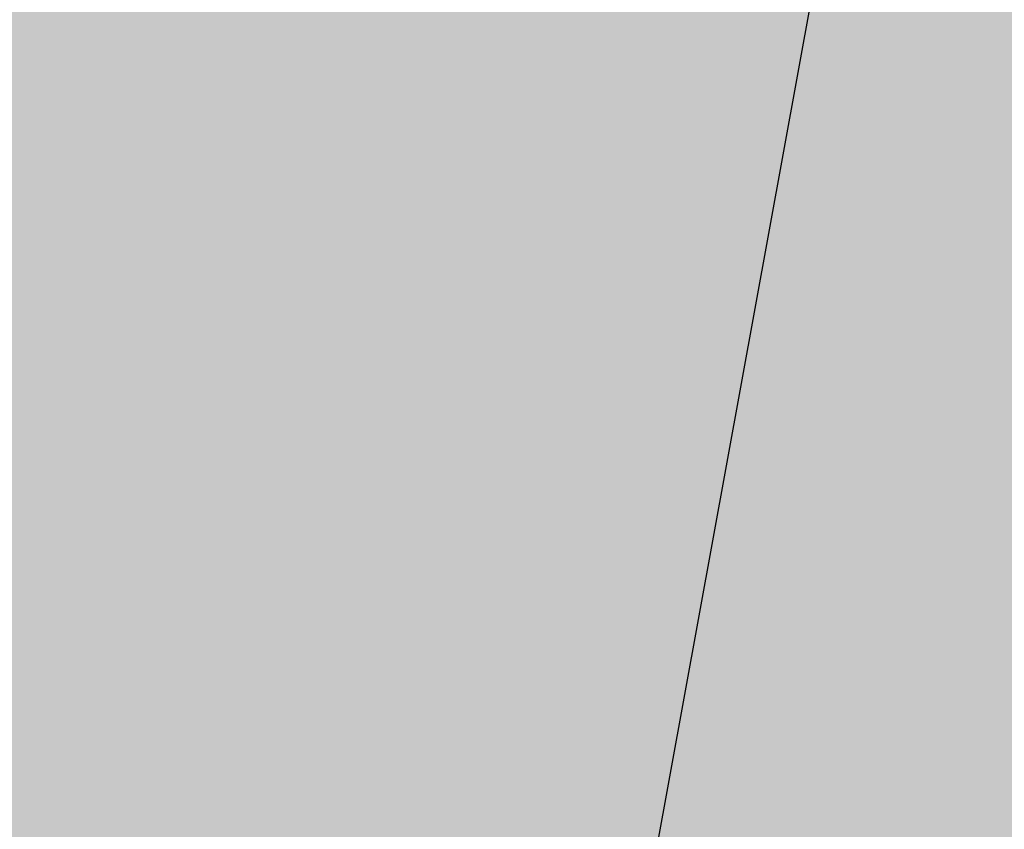
# Model space of a CAD drawing. Units: feet. Extents: x 3168 to 4724, y 827 to 1477.
# Tile 237 of 256: x 3382.882 to 3384.783, y 1096.781 to 1098.344. Entities that reach past the tile are written whole.
import ezdxf

# ---------------------------------------------------------------- set-up
doc = ezdxf.new("R2010")
doc.units = ezdxf.units.FT
doc.layers.add('A-ELEV-PATT', color=8, linetype='Continuous', lineweight=13)
doc.layers.add('C-TOPO', color=3, linetype='Continuous', lineweight=25)

msp = doc.modelspace()

# ---------------------------------------------------------------- hatches: boundary and pattern name
at = {"layer": 'A-ELEV-PATT'}
h = msp.add_hatch(color=256, dxfattribs=at)
h.dxf.hatch_style = 1
edge = h.paths.add_edge_path()
edge.add_ellipse((3552.9058, 979.2201), major_axis=(36.7449, 0), ratio=0.4848485, start_angle=0, end_angle=360)
edge = h.paths.add_edge_path()
edge.add_ellipse((3559.8916, 929.2523), major_axis=(36.7449, 0), ratio=0.4848485, start_angle=0, end_angle=360)
edge = h.paths.add_edge_path()
edge.add_line((3299.3168, 1198.6061), (3479.9167, 1198.6061))
edge.add_line((3479.9167, 1198.6061), (3479.9167, 1209.8686))
edge.add_spline(control_points=[(3479.9167, 1209.8686), (3464.3012, 1209.8686), (3448.6856, 1209.8686), (3410.9491, 1209.8686), (3388.8282, 1209.8686), (3355.6469, 1209.8686), (3344.5864, 1209.8686), (3327.9957, 1209.8686), (3322.4655, 1209.8686), (3314.1702, 1209.8686), (3311.4051, 1209.8686), (3307.2574, 1209.8686), (3305.8748, 1209.8686), (3303.801, 1209.8686), (3303.1097, 1209.8686), (3302.0728, 1209.8686), (3301.7272, 1209.8686), (3301.2087, 1209.8686), (3301.0359, 1209.8686), (3300.7767, 1209.8686), (3300.6903, 1209.8686), (3300.5606, 1209.8686), (3300.5174, 1209.8686), (3300.4526, 1209.8686), (3300.431, 1209.8686), (3300.3986, 1209.8686), (3300.3878, 1209.8686), (3300.3662, 1209.8686), (3300.3457, 1209.8686), (3300.3455, 1209.8686), (3300.3455, 1209.8686), (3300.3433, 1209.8686), (3300.3411, 1209.8686), (3300.3379, 1209.8686), (3300.3368, 1209.8686), (3300.3339, 1209.8686), (3300.3321, 1209.8686), (3300.3255, 1209.8686), (3300.3207, 1209.8686), (3300.3109, 1209.8686), (3300.306, 1209.8686), (3300.2905, 1209.8686), (3300.28, 1209.8686), (3300.2324, 1209.8688), (3300.1953, 1209.869), (3299.9511, 1209.8706), (3299.7448, 1209.8743), (3299.4368, 1209.8833), (3299.3344, 1209.8868), (3299.1811, 1209.8929), (3299.13, 1209.8951), (3298.6522, 1209.9168), (3298.2295, 1209.9457), (3297.6016, 1210.0024), (3297.3934, 1210.0235), (3297.0827, 1210.0583), (3296.9793, 1210.0705), (3296.293, 1210.1549), (3295.7181, 1210.2434), (3294.8687, 1210.3989), (3294.5877, 1210.4545), (3294.1693, 1210.5433), (3294.0304, 1210.5739), (3291.7071, 1211.1012), (3289.6536, 1211.8134), (3285.7763, 1213.564), (3283.9514, 1214.6035), (3280.5122, 1216.9801), (3278.8972, 1218.3176), (3276.3799, 1220.8295), (3275.416, 1221.9177), (3274.0393, 1223.7077), (3273.581, 1224.3495), (3273.1432, 1225.0163)], knot_values=[39.119033, 39.119033, 39.119033, 39.119033, 39.286353, 39.286353, 39.523379, 39.523379, 39.641892, 39.641892, 39.701148, 39.701148, 39.730777, 39.730777, 39.745591, 39.745591, 39.752998, 39.752998, 39.756701, 39.756701, 39.758553, 39.758553, 39.759479, 39.759479, 39.759942, 39.759942, 39.760173, 39.760173, 39.760289, 39.760289, 39.760405, 39.760405, 39.760463, 39.760463, 39.763389, 39.763389, 39.764851, 39.764851, 39.767304, 39.767304, 39.773825, 39.773825, 39.78057, 39.78057, 39.79477, 39.79477, 39.845194, 39.845194, 40.126715, 40.126715, 40.267476, 40.267476, 40.337856, 40.337856, 40.927023, 40.927023, 41.221606, 41.221606, 41.368898, 41.368898, 42.202622, 42.202622, 42.619485, 42.619485, 42.827916, 42.827916, 46.118323, 46.118323, 49.408731, 49.408731, 52.699139, 52.699139, 54.927489, 54.927489, 56.104228, 56.104228, 56.104228, 56.104228], weights=[1, 1, 1, 1, 1, 1, 1, 1, 1, 1, 1, 1, 1, 1, 1, 1, 1, 1, 1, 1, 1, 1, 1, 1, 1, 1, 1, 1, 1, 1, 1, 1, 1, 1, 1, 1, 1, 1, 1, 1, 1, 1, 1, 1, 1, 1, 1, 1, 1, 1, 1, 1, 1, 1, 1, 1, 1, 1, 1, 1, 1, 1, 1, 1, 1, 1, 1, 1, 1, 1, 1, 1, 1, 1], degree=3, periodic=0)
edge.add_line((3273.1432, 1225.0163), (3273.1432, 1099.0163))
edge.add_line((3273.1432, 1099.0163), (3299.3168, 1099.0163))
edge.add_line((3299.3168, 1099.0163), (3299.3168, 1198.6061))
edge = h.paths.add_edge_path()
edge.add_line((3304.7584, 1324.1581), (3479.9167, 1324.1581))
edge.add_line((3479.9167, 1324.1581), (3479.9167, 1335.7146))
edge.add_line((3479.9167, 1335.7146), (3269.1616, 1335.7146))
edge.add_spline(control_points=[(3269.1616, 1335.7146), (3264.0242, 1335.7146), (3258.3641, 1328.9582), (3259.2643, 1323.9003)], knot_values=[0, 0, 0, 0, 15.412191, 15.412191, 15.412191, 15.412191], degree=3, periodic=0)
edge.add_line((3259.2643, 1323.9003), (3265.5168, 1288.7691))
edge.add_line((3265.5168, 1288.7691), (3275.2651, 1261.5456))
edge.add_line((3275.2651, 1261.5456), (3304.7584, 1261.5456))
edge.add_line((3304.7584, 1261.5456), (3304.7584, 1324.1581))
h = msp.add_hatch(color=256, dxfattribs=at)
h.dxf.hatch_style = 1
h.paths.add_polyline_path([(3384.5252, 1099.0163), (3335.0292, 1099.0163), (3299.3168, 1099.0163), (3273.1432, 1099.0163), (3217.5654, 1099.0163), (3168.0693, 827.1163), (3335.0292, 827.1163)])
h = msp.add_hatch(color=256, dxfattribs=at)
h.dxf.hatch_style = 1
h.paths.add_polyline_path([(3845.3757, 1099.0163), (3706.2884, 1099.0163), (3715.6187, 1081.3955), (3715.6187, 1052.3102), (3792.0552, 907.9557), (3463.2221, 903.6425), (3462.8992, 928.2574, 0.540152), (3462.8992, 1014.0826), (3621.8987, 1014.0826), (3601.657, 1052.3102), (3601.657, 1081.3955), (3592.3267, 1099.0163), (3384.5252, 1099.0163), (3335.0292, 827.1163), (3845.3757, 827.1163)])

# ---------------------------------------------------------------- linework, layer by layer
at = {"layer": 'C-TOPO'}
msp.add_line((3384.5252, 1099.0163), (3335.0292, 827.1163), dxfattribs=at)
msp.add_lwpolyline([(3384.5252, 1099.0163), (3335.0292, 827.1163), (3845.3757, 827.1163), (3845.3757, 1099.0163), (3335.0292, 1099.0163)], dxfattribs=at)

doc.saveas('drawing.dxf')
